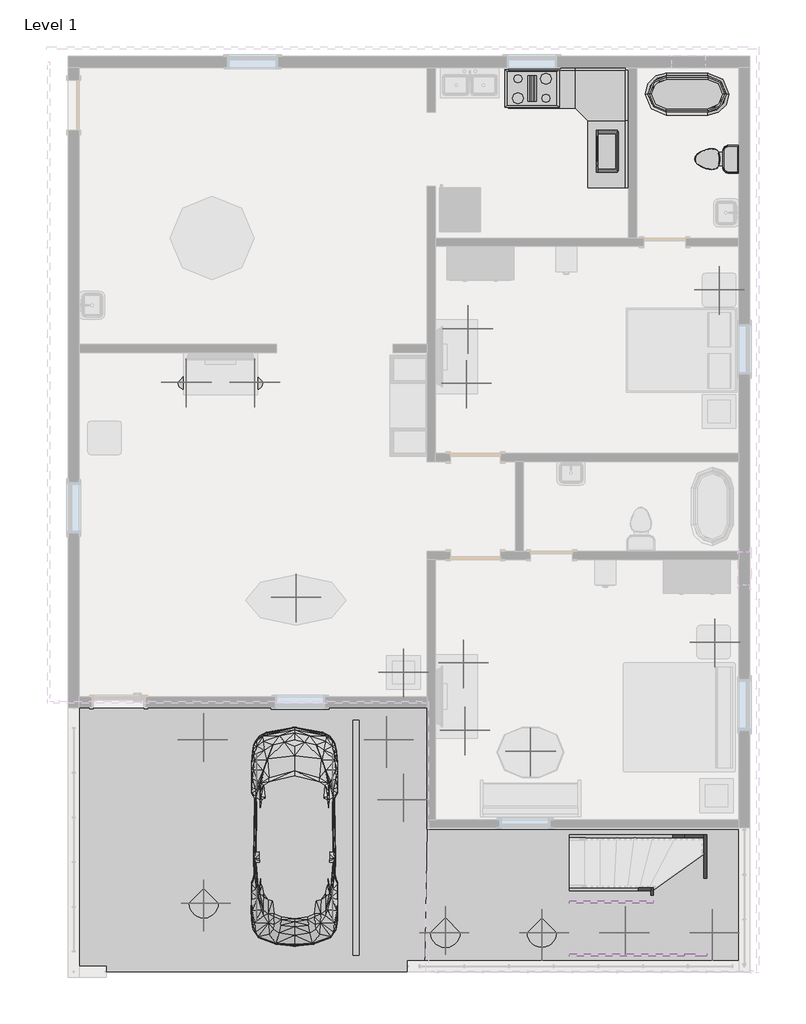
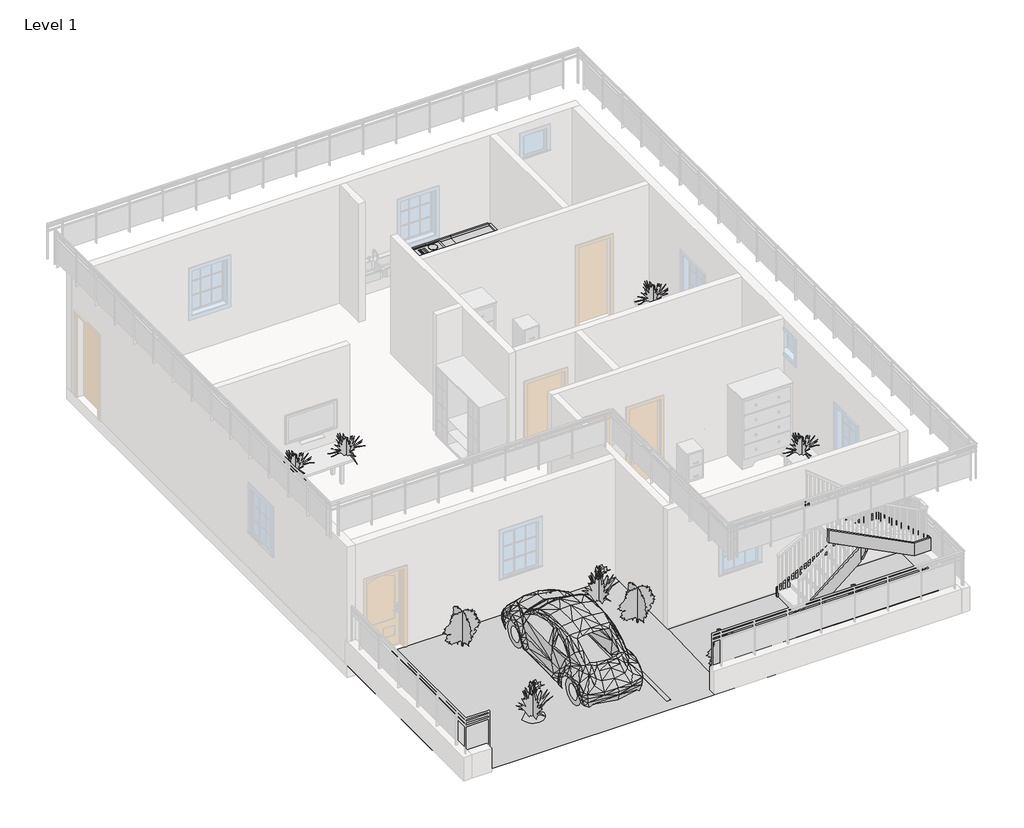
# One storey, part 5 of 5: 19 geographic elements, 8 members, 6 proxies, 3 flow terminals, 1 furniture element.
"""IFC4 building model written with IfcOpenShell, lengths in millimetres."""

from ifc_helpers import new_model, si_unit, frame, origin, place, context, project, spatial, polyline, outline, extrude, triangles, transform, mapped, element, save
from components import proxy_bb1e6e30, proxy_8a8d5ab2, parking_space_9_x_18_90_deg_fdd9e8f5, rpc_beetle_rpc_beetle_3ce7ba48, flow_terminal_accce45a, toilet_domestic_3d_toilet_domestic_3d_f7549cf7, toilet_domestic_3d_toilet_domestic_3d_183bbd19, flow_terminal_b374fae2, furniture_4f0cce40, rpc_plant_tropical_55f6ff97, rpc_plant_tropical_agave_1_5_93a2a214, rpc_plant_tropical_jungle_flame_3_9c4808c2

model = new_model("IFC4")

# Units and contexts
model_context = context("Model", 3, world=origin())
ifc_project = project(units=[si_unit("LENGTHUNIT", "METRE", prefix="MILLI")], contexts=[model_context])

# Site, building, storey
site = spatial("IfcSite", under=ifc_project)
building = spatial("IfcBuilding", under=site)
storey = spatial("IfcBuildingStorey", under=building, Name="Level 1", Elevation=0.0)

# Proxies
placement = place(None, origin())
element("IfcBuildingElementProxy", 1, Name="Building Element Proxy", at=placement, inside=storey, context=model_context, shape_type="Tessellation", body=[
    triangles([(-5791.023848, -19.9366942, 0.0), (-5841.8242355, -2636.1367676, 0.0), (76.3758886, -19.9366942, 0.0), (76.3758886, -2636.1367676, 0.0)], [[1, 2, 4], [4, 3, 1]], closed=False),
])
element("IfcBuildingElementProxy", 2, Name="Building Element Proxy", at=placement, inside=storey, context=model_context, shape_type="Tessellation", body=[
    triangles([(-12318.8236542, 2164.4633778, 0.0), (-12318.8236542, -2636.1367676, 0.0), (-5841.8242355, -2636.1367676, 0.0), (-5791.023848, 2164.4633778, 0.0), (-5791.023848, -19.9366942, 0.0)], [[1, 2, 5], [5, 4, 1], [5, 2, 3]], closed=False),
])
proxy_shape = proxy_bb1e6e30(model_context)
element("IfcBuildingElementProxy", 3, Name="Cook Top-4 Unit : 36\" x 20\"", ObjectType="Cook Top-4 Unit : 36\" x 20\"", at=placement, inside=storey, context=model_context, shape_type="MappedRepresentation", body=[
    mapped(proxy_shape, transform((-3886.0241134, 13416.6633056, 0.0), x_axis=(1.0, 0.0, 0.0), y_axis=(0.0, 1.0, 0.0), z_axis=(0.0, 0.0, 1.0))),
])
proxy_2_shape = proxy_8a8d5ab2(model_context)
element("IfcBuildingElementProxy", 4, Name="Microwave : 30\" x 16\" x 18\"", ObjectType="Microwave : 30\" x 16\" x 18\"", at=placement, inside=storey, context=model_context, shape_type="MappedRepresentation", body=[
    mapped(proxy_2_shape, transform((-2161.3436076, 12773.956183, 0.0), x_axis=(0.0, -1.0000000000000004, 0.0), y_axis=(1.0000000000000004, 0.0, 0.0), z_axis=(0.0, 0.0, 1.0))),
])
parking_space_9_x_18_90_deg_shape = parking_space_9_x_18_90_deg_fdd9e8f5(model_context)
element("IfcBuildingElementProxy", 5, Name="Parking Space : 9' x 18' - 90 deg", ObjectType="Parking Space : 9' x 18' - 90 deg", at=placement, inside=storey, context=model_context, shape_type="MappedRepresentation", body=[
    mapped(parking_space_9_x_18_90_deg_shape, transform((-7086.4241134, -2331.3366944, 0.0), x_axis=(-0.9999999999999999, 0.0, 0.0), y_axis=(0.0, -0.9999999999999999, 0.0), z_axis=(0.0, 0.0, 1.0))),
])
rpc_beetle_rpc_beetle_shape = rpc_beetle_rpc_beetle_3ce7ba48(model_context)
element("IfcBuildingElementProxy", 6, Name="RPC Beetle : RPC Beetle", ObjectType="RPC Beetle : RPC Beetle", at=placement, inside=storey, context=model_context, shape_type="MappedRepresentation", body=[
    mapped(rpc_beetle_rpc_beetle_shape, transform((-8204.0241134, -1416.9366944, 0.0), x_axis=(1.0, 0.0, 0.0), y_axis=(0.0, 1.0, 0.0), z_axis=(0.0, 0.0, 1.0))),
])

# Flow terminals
flow_terminal_shape = flow_terminal_accce45a(model_context)
element("IfcFlowTerminal", 7, ObjectType="Floor Drain - Round : 5\" Strainer - 2\" Drain", at=placement, inside=storey, context=model_context, shape_type="MappedRepresentation", body=[
    mapped(flow_terminal_shape, transform((-412.5741134, 12654.6633056, 0.0), x_axis=(1.0, 0.0, 0.0), y_axis=(0.0, 1.0, 0.0), z_axis=(0.0, 0.0, 1.0))),
])
toilet_domestic_3d_toilet_domestic_3d_shape = toilet_domestic_3d_toilet_domestic_3d_f7549cf7(model_context)
toilet_domestic_3d_toilet_domestic_3d_2_shape = toilet_domestic_3d_toilet_domestic_3d_183bbd19(model_context)
element("IfcFlowTerminal", 8, ObjectType="Toilet-Domestic-3D : Toilet-Domestic-3D", at=placement, inside=storey, context=model_context, shape_type="MappedRepresentation", body=[
    mapped(toilet_domestic_3d_toilet_domestic_3d_shape, transform((-621.5201408, 12133.9633056, 0.0), x_axis=(0.0, -1.0000000000000004, 0.0), y_axis=(1.0000000000000004, 0.0, 0.0), z_axis=(0.0, 0.0, 1.0))),
    mapped(toilet_domestic_3d_toilet_domestic_3d_2_shape, transform((-621.5201408, 12133.9633056, 0.0), x_axis=(0.0, -1.0000000000000004, 0.0), y_axis=(1.0000000000000004, 0.0, 0.0), z_axis=(0.0, 0.0, 1.0))),
])
flow_terminal_2_shape = flow_terminal_b374fae2(model_context)
element("IfcFlowTerminal", 9, ObjectType="Tub-Free Standing-3D : 30\" x 60\"", at=placement, inside=storey, context=model_context, shape_type="MappedRepresentation", body=[
    mapped(flow_terminal_2_shape, transform((-1066.6241134, 13315.0633056, 0.0), x_axis=(0.0, 1.0000000000000002, 0.0), y_axis=(-1.0000000000000002, 0.0, 0.0), z_axis=(0.0, 0.0, 1.0))),
])

# Furniture
furniture_shape = furniture_4f0cce40(model_context)
element("IfcFurniture", 10, ObjectType="Work Station Cubicle : 96\" x 96\"", at=placement, inside=storey, context=model_context, shape_type="MappedRepresentation", body=[
    mapped(furniture_shape, transform((-1638.4011058, 13665.9315534, 0.0), x_axis=(0.0, -1.0000000000000004, 0.0), y_axis=(1.0000000000000004, 0.0, 0.0), z_axis=(0.0, 0.0, 1.0))),
])

# Geographic elements
rpc_plant_tropical_shape = rpc_plant_tropical_55f6ff97(model_context)
element("IfcGeographicElement", 11, ObjectType="RPC Plant - Tropical", at=placement, inside=storey, context=model_context, shape_type="MappedRepresentation", body=[
    mapped(rpc_plant_tropical_shape, transform((-6527.6241134, 1580.2633056, 0.0), x_axis=(1.0, 0.0, 0.0), y_axis=(0.0, 1.0, 0.0), z_axis=(0.0, 0.0, 1.0))),
])
element("IfcGeographicElement", 12, ObjectType="RPC Plant - Tropical", at=placement, inside=storey, context=model_context, shape_type="MappedRepresentation", body=[
    mapped(rpc_plant_tropical_shape, transform((-609.4241134, -1924.9366944, 0.0), x_axis=(1.0, 0.0, 0.0), y_axis=(0.0, 1.0, 0.0), z_axis=(0.0, 0.0, 1.0))),
])
element("IfcGeographicElement", 13, ObjectType="RPC Plant - Tropical", at=placement, inside=storey, context=model_context, shape_type="MappedRepresentation", body=[
    mapped(rpc_plant_tropical_shape, transform((-3708.2241134, -1924.9366944, 0.0), x_axis=(1.0, 0.0, 0.0), y_axis=(0.0, 1.0, 0.0), z_axis=(0.0, 0.0, 1.0))),
])
element("IfcGeographicElement", 14, ObjectType="RPC Plant - Tropical", at=placement, inside=storey, context=model_context, shape_type="MappedRepresentation", body=[
    mapped(rpc_plant_tropical_shape, transform((-9855.0241134, -1391.5366944, 0.0), x_axis=(1.0, 0.0, 0.0), y_axis=(0.0, 1.0, 0.0), z_axis=(0.0, 0.0, 1.0))),
])
rpc_plant_tropical_agave_1_5_shape = rpc_plant_tropical_agave_1_5_93a2a214(model_context)
element("IfcGeographicElement", 15, ObjectType="RPC Plant - Tropical : Agave - 1.5'", at=placement, inside=storey, context=model_context, shape_type="MappedRepresentation", body=[
    mapped(rpc_plant_tropical_agave_1_5_shape, transform((-482.4241134, 9759.0633056, 609.6), x_axis=(1.0, 0.0, 0.0), y_axis=(0.0, 1.0, 0.0), z_axis=(0.0, 0.0, 1.0))),
])
element("IfcGeographicElement", 16, ObjectType="RPC Plant - Tropical : Agave - 1.5'", at=placement, inside=storey, context=model_context, shape_type="MappedRepresentation", body=[
    mapped(rpc_plant_tropical_agave_1_5_shape, transform((-5054.4241134, 9047.8633056, 609.6), x_axis=(1.0, 0.0, 0.0), y_axis=(0.0, 1.0, 0.0), z_axis=(0.0, 0.0, 1.0))),
])
element("IfcGeographicElement", 17, ObjectType="RPC Plant - Tropical : Agave - 1.5'", at=placement, inside=storey, context=model_context, shape_type="MappedRepresentation", body=[
    mapped(rpc_plant_tropical_agave_1_5_shape, transform((-5079.8241134, 8057.2633056, 609.6), x_axis=(1.0, 0.0, 0.0), y_axis=(0.0, 1.0, 0.0), z_axis=(0.0, 0.0, 1.0))),
])
element("IfcGeographicElement", 18, ObjectType="RPC Plant - Tropical : Agave - 1.5'", at=placement, inside=storey, context=model_context, shape_type="MappedRepresentation", body=[
    mapped(rpc_plant_tropical_agave_1_5_shape, transform((-558.6241134, 3358.2633056, 609.6), x_axis=(1.0, 0.0, 0.0), y_axis=(0.0, 1.0, 0.0), z_axis=(0.0, 0.0, 1.0))),
])
element("IfcGeographicElement", 19, ObjectType="RPC Plant - Tropical : Agave - 1.5'", at=placement, inside=storey, context=model_context, shape_type="MappedRepresentation", body=[
    mapped(rpc_plant_tropical_agave_1_5_shape, transform((-5130.6241134, 2977.2633056, 660.4), x_axis=(1.0, 0.0, 0.0), y_axis=(0.0, 1.0, 0.0), z_axis=(0.0, 0.0, 1.0))),
])
element("IfcGeographicElement", 20, ObjectType="RPC Plant - Tropical : Agave - 1.5'", at=placement, inside=storey, context=model_context, shape_type="MappedRepresentation", body=[
    mapped(rpc_plant_tropical_agave_1_5_shape, transform((-5105.2241134, 1758.0633056, 660.4), x_axis=(1.0, 0.0, 0.0), y_axis=(0.0, 1.0, 0.0), z_axis=(0.0, 0.0, 1.0))),
])
element("IfcGeographicElement", 21, ObjectType="RPC Plant - Tropical : Agave - 1.5'", at=placement, inside=storey, context=model_context, shape_type="MappedRepresentation", body=[
    mapped(rpc_plant_tropical_agave_1_5_shape, transform((-3911.4241134, 1377.0633056, 736.6), x_axis=(1.0, 0.0, 0.0), y_axis=(0.0, 1.0, 0.0), z_axis=(0.0, 0.0, 1.0))),
])
element("IfcGeographicElement", 22, ObjectType="RPC Plant - Tropical : Agave - 1.5'", at=placement, inside=storey, context=model_context, shape_type="MappedRepresentation", body=[
    mapped(rpc_plant_tropical_agave_1_5_shape, transform((-6222.8241134, 2805.8133056, 609.6), x_axis=(1.0, 0.0, 0.0), y_axis=(0.0, 1.0, 0.0), z_axis=(0.0, 0.0, 1.0))),
])
element("IfcGeographicElement", 23, ObjectType="RPC Plant - Tropical : Agave - 1.5'", at=placement, inside=storey, context=model_context, shape_type="MappedRepresentation", body=[
    mapped(rpc_plant_tropical_agave_1_5_shape, transform((-8178.6241134, 4171.0633056, 685.8), x_axis=(1.0, 0.0, 0.0), y_axis=(0.0, 1.0, 0.0), z_axis=(0.0, 0.0, 1.0))),
])
element("IfcGeographicElement", 24, ObjectType="RPC Plant - Tropical : Agave - 1.5'", at=placement, inside=storey, context=model_context, shape_type="MappedRepresentation", body=[
    mapped(rpc_plant_tropical_agave_1_5_shape, transform((-8927.9241134, 8082.6633056, 660.4), x_axis=(1.0, 0.0, 0.0), y_axis=(0.0, 1.0, 0.0), z_axis=(0.0, 0.0, 1.0))),
])
element("IfcGeographicElement", 25, ObjectType="RPC Plant - Tropical : Agave - 1.5'", at=placement, inside=storey, context=model_context, shape_type="MappedRepresentation", body=[
    mapped(rpc_plant_tropical_agave_1_5_shape, transform((-10172.5241134, 8082.6633056, 660.4), x_axis=(1.0, 0.0, 0.0), y_axis=(0.0, 1.0, 0.0), z_axis=(0.0, 0.0, 1.0))),
])
rpc_plant_tropical_jungle_flame_3_shape = rpc_plant_tropical_jungle_flame_3_9c4808c2(model_context)
element("IfcGeographicElement", 26, ObjectType="RPC Plant - Tropical : Jungle Flame - 3'", at=placement, inside=storey, context=model_context, shape_type="MappedRepresentation", body=[
    mapped(rpc_plant_tropical_jungle_flame_3_shape, transform((-6222.8241134, 488.0633056, 0.0), x_axis=(1.0, 0.0, 0.0), y_axis=(0.0, 1.0, 0.0), z_axis=(0.0, 0.0, 1.0))),
])
element("IfcGeographicElement", 27, ObjectType="RPC Plant - Tropical : Jungle Flame - 3'", at=placement, inside=storey, context=model_context, shape_type="MappedRepresentation", body=[
    mapped(rpc_plant_tropical_jungle_flame_3_shape, transform((-2184.2241134, -1924.9366944, 0.0), x_axis=(1.0, 0.0, 0.0), y_axis=(0.0, 1.0, 0.0), z_axis=(0.0, 0.0, 1.0))),
])
element("IfcGeographicElement", 28, ObjectType="RPC Plant - Tropical : Jungle Flame - 3'", at=placement, inside=storey, context=model_context, shape_type="MappedRepresentation", body=[
    mapped(rpc_plant_tropical_jungle_flame_3_shape, transform((-5460.8241134, -1924.9366944, 0.0), x_axis=(1.0, 0.0, 0.0), y_axis=(0.0, 1.0, 0.0), z_axis=(0.0, 0.0, 1.0))),
])
element("IfcGeographicElement", 29, ObjectType="RPC Plant - Tropical : Jungle Flame - 3'", at=placement, inside=storey, context=model_context, shape_type="MappedRepresentation", body=[
    mapped(rpc_plant_tropical_jungle_flame_3_shape, transform((-9855.0241134, 1580.2633056, 0.0), x_axis=(1.0, 0.0, 0.0), y_axis=(0.0, 1.0, 0.0), z_axis=(0.0, 0.0, 1.0))),
])

# Members
element("IfcMember", 30, ObjectType="Stringer - 2\" Width", at=placement, inside=storey, context=model_context, shape_type="SweptSolid", body=[
    extrude(outline(polyline([(229.639954, -3203.9558053), (0.0, -3203.9558053), (0.0, -2984.1934877), (962.500629, -1116.5386136), (1305.3956453, -1116.5386136), (229.639954, -3203.9558053)])), frame((0.0, -197.7366944, 0.0), z_axis=(0.0, 1.0, 0.0), x_axis=(0.0, 0.0, 1.0)), (0.0, 0.0, 1.0), 50.8),
])
element("IfcMember", 31, ObjectType="Stringer - 2\" Width", at=placement, inside=storey, context=model_context, shape_type="SweptSolid", body=[
    extrude(outline(polyline([(-1116.5386136, -197.7366944), (-1116.5386136, -146.9366944), (-761.8241134, -146.9366944), (-761.8241134, -197.7366944), (-1116.5386136, -197.7366944)])), frame((0.0, 0.0, 962.500629), z_axis=(0.0, 0.0, 1.0), x_axis=(1.0, 0.0, 0.0)), (0.0, 0.0, 1.0), 342.8950162),
])
element("IfcMember", 32, ObjectType="Stringer - 2\" Width", at=placement, inside=storey, context=model_context, shape_type="SweptSolid", body=[
    extrude(outline(polyline([(-146.9366944, 1289.0952212), (-146.9366944, 1000.5956453), (-316.4591773, 1000.5956453), (-2305.9366944, 1638.9682298), (-2305.9366944, 1969.9972697), (-2268.9565771, 1969.9972697), (-146.9366944, 1289.0952212)])), frame((-761.8241134, 0.0, 0.0), z_axis=(1.0, 0.0, 0.0), x_axis=(0.0, 1.0, 0.0)), (0.0, 0.0, 1.0), 50.8),
])
element("IfcMember", 33, ObjectType="Stringer - 2\" Width", at=placement, inside=storey, context=model_context, shape_type="SweptSolid", body=[
    extrude(outline(polyline([(-711.0241134, -2305.9366944), (-711.0241134, -2356.7366944), (-1116.5386136, -2356.7366944), (-1116.5386136, -2305.9366944), (-711.0241134, -2305.9366944)])), frame((0.0, 0.0, 1649.8904473), z_axis=(0.0, 0.0, 1.0), x_axis=(1.0, 0.0, 0.0)), (0.0, 0.0, 1.0), 320.1068224),
])
element("IfcMember", 34, ObjectType="Stringer - 2\" Width", at=placement, inside=storey, context=model_context, shape_type="SweptSolid", body=[
    extrude(outline(polyline([(1649.8904473, -1116.5386136), (1969.9972697, -1116.5386136), (3045.7529609, -3203.9558053), (2725.6461385, -3203.9558053), (1649.8904473, -1116.5386136)])), frame((0.0, -2356.7366944, 0.0), z_axis=(0.0, 1.0, 0.0), x_axis=(0.0, 0.0, 1.0)), (0.0, 0.0, 1.0), 50.8),
])
element("IfcMember", 35, ObjectType="Stringer - 2\" Width", at=placement, inside=storey, context=model_context, shape_type="SweptSolid", body=[
    extrude(outline(polyline([(176.1764461, -3203.9558053), (0.0, -3203.9558053), (0.0, -2937.6941607), (987.1410923, -1727.0241134), (1380.418648, -1727.0241134), (176.1764461, -3203.9558053)])), frame((0.0, -1162.9366944, 0.0), z_axis=(0.0, 1.0, 0.0), x_axis=(0.0, 0.0, 1.0)), (0.0, 0.0, 1.0), 50.8),
])
element("IfcMember", 36, ObjectType="Stringer - 2\" Width", at=placement, inside=storey, context=model_context, shape_type="SweptSolid", body=[
    extrude(outline(polyline([(-1112.1366944, 1573.2682978), (-1112.1366944, 1028.5617647), (-1146.3789117, 1028.5617647), (-1340.7366944, 1360.465107), (-1340.7366944, 1926.1409689), (-1318.7738118, 1926.1409689), (-1112.1366944, 1573.2682978)])), frame((-1727.0241134, 0.0, 0.0), z_axis=(1.0, 0.0, 0.0), x_axis=(0.0, 1.0, 0.0)), (0.0, 0.0, 1.0), 50.8),
])
element("IfcMember", 37, ObjectType="Stringer - 2\" Width", at=placement, inside=storey, context=model_context, shape_type="SweptSolid", body=[
    extrude(outline(polyline([(1532.8634131, -1676.2241134), (1926.1409689, -1676.2241134), (3171.8038432, -3203.9558053), (2778.5262875, -3203.9558053), (1532.8634131, -1676.2241134)])), frame((0.0, -1391.5366944, 0.0), z_axis=(0.0, 1.0, 0.0), x_axis=(0.0, 0.0, 1.0)), (0.0, 0.0, 1.0), 50.8),
])

save(model, "model.ifc")

# Revit data of these elements
# Type "Cook Top-4 Unit : 36\" x 20\""
#   Assembly Code = "E1090400"
#   Depth = 2' - 0"
#   Width = 3' - 0"
#   Burner Material = Steel, Chrome Plated
#   Cooktop Material = Steel, Polished
#   Default Elevation = 0
# Type "Microwave : 30\" x 16\" x 18\""
#   Assembly Code = "E1090400"
#   Depth = 1' - 4"
#   Height = 1' - 6"
#   Width = 2' - 6"
#   Microwave Material = Laminate, Linen, Matte
#   Default Elevation = 0
# Type "Parking Space : 9' x 18' - 90 deg"
#   Angle = 90.00°
#   Parking Length = 18' - 0"
#   Parking Width = 9' - 0"
#   pl = 14' - 0"
#   pw = 7' - 0"
# Type "RPC Beetle : RPC Beetle"
#   built-in parameter 1005195 = "RPC-16-0U6E-L4EG-ENH1-J3KF-SVEL-0TX4-C0"
#   Height = 0
# Type "Floor Drain - Round : 5\" Strainer - 2\" Drain"
#   WFU = 2
#   Strainer Height = 0' - 3 1/4"
#   Strainer Radius = 0' - 2 1/2"
#   Strainer Diameter = 0' - 5"
#   Radius 6 = 0' - 0 5/8"
#   Radius 5 = 0' - 1 1/4"
#   Radius 4 = 0' - 1 7/8"
#   Radius 2 = 0' - 3.04167"
#   Radius 1 = 0' - 2.02083"
#   Radius 3 = 0' - 2 1/32"
#   Pipe Radius = 1"
#   Pipe Diameter = 2"
#   Height 2 = 0' - 0.725"
#   Height 1 = 0' - 1 13/16"
#   Body Radius = 0' - 4 1/16"
#   Body Height = 0' - 3 5/8"
#   Body Diameter = 0' - 8 1/8"
#   Drain Material = none
#   HWFU = 0
#   Default Elevation = 0
#   CWFU = 0
# Type "Toilet-Domestic-3D : Toilet-Domestic-3D"
#   Assembly Code = "D2010110"
#   Toilet - Bowl/Basin Material = Porcelain, Linen
#   Toilet - Seat Material = Laminate, Linen, Matte
#   Default Elevation = 0
# Type "Tub-Free Standing-3D : 30\" x 60\""
#   Assembly Code = "D2010110"
#   Height = 1' - 6"
#   Length = 5' - 0"
#   Width = 2' - 6"
#   Tub Material = Porcelain, Ivory
#   Default Elevation = 0
# Type "Work Station Cubicle : 96\" x 96\""
#   Assembly Code = "E2020"
#   Desktop Height = 2' - 6"
#   Desktop1 Width = 2' - 3"
#   Desktop2 Width = 2' - 3"
#   Panel Height = 2' - 8"
#   Panel1 Length = 4' - 0"
#   Panel2 Length = 4' - 0"
#   Cube Panel Material = Textile - Light Gray
#   Work Top Material = Laminate, Ivory, Matte
#   Default Elevation = 0
# Type "RPC Plant - Tropical"
#   built-in parameter 1005198 = "{2, 15},{39, RPC-16-FWM5-GM7X-C67P-4000-ST1L-LVER-AU},{1, 0},{1, 0},{2, 13},{1, 8},{5, Color},{1, 0},{1, 0},{3, 0.8},{3, 0.8},{3, 0.8},{1, 8},{7, BBoxMin},{1, 0},{1, 0},{1, 0},{1, 0},{1, 0},{1, 8},{7, BBoxMax},{1, 0},{1, 0},{1, 0},{1, 0},{1, 0},{2, 11},{9, RPCTypeId},{1, 0},{1, 0},{39, RPC-16-FWM5-GM7X-C67P-4000-ST1L-LVER-AU},{1, 6},{14, RPCPlantHeight},{1, 0},{1, 0},{1, 3},{2, 11},{7, keyword},{1, 0},{1, 0},{35, :RPCs:Shrubs [General]:Geometry:RPC},{2, 11},{8, category},{1, 0},{1, 0},{16, Shrubs [General]},{2, 11},{12, LocalizedUID},{1, 0},{1, 0},{10, Crane Lily},{2, 14},{6, Height},{1, 0},{1, 0},{1, 3},{1, 2},{16, Cast Reflections},{1, 0},{1, 0},{1, 0},{1, 2},{12, Cast Shadows},{1, 0},{1, 0},{1, 1},{1, 2},{9, Lock View},{1, 0},{1, 0},{1, 0},{1, 4},{5, ViewC},{1, 0},{1, 0},{1, 0},{21, assetlibrary_base.fbx},{1, 5},"
#   built-in parameter 1005195 = "RPC-16-FWM5-GM7X-C67P-4000-ST1L-LVER-AU"
#   Assembly Code = "G2050500"
#   Height = 3' - 0"
#   Default Elevation = 0
# Type "RPC Plant - Tropical : Agave - 1.5'"
#   built-in parameter 1005198 = "{2, 15},{39, RPC-16-G1GJ-63FX-7K5P-N000-ST1L-LVER-AU},{1, 0},{1, 0},{2, 13},{1, 8},{5, Color},{1, 0},{1, 0},{3, 0.8},{3, 0.8},{3, 0.8},{1, 8},{7, BBoxMin},{1, 0},{1, 0},{1, 0},{1, 0},{1, 0},{1, 8},{7, BBoxMax},{1, 0},{1, 0},{1, 0},{1, 0},{1, 0},{2, 11},{9, RPCTypeId},{1, 0},{1, 0},{39, RPC-16-G1GJ-63FX-7K5P-N000-ST1L-LVER-AU},{1, 6},{14, RPCPlantHeight},{1, 0},{1, 0},{3, 1.5},{2, 11},{7, keyword},{1, 0},{1, 0},{35, :RPCs:Plants [General]:Geometry:RPC},{2, 11},{8, category},{1, 0},{1, 0},{16, Plants [General]},{2, 11},{12, LocalizedUID},{1, 0},{1, 0},{5, Agave},{2, 14},{6, Height},{1, 0},{1, 0},{3, 1.5},{1, 2},{16, Cast Reflections},{1, 0},{1, 0},{1, 0},{1, 2},{12, Cast Shadows},{1, 0},{1, 0},{1, 1},{1, 2},{9, Lock View},{1, 0},{1, 0},{1, 0},{1, 4},{5, ViewC},{1, 0},{1, 0},{1, 0},{21, assetlibrary_base.fbx},{1, 5},"
#   built-in parameter 1005195 = "RPC-16-G1GJ-63FX-7K5P-N000-ST1L-LVER-AU"
#   Type Comments = "Agave"
#   Assembly Code = "G2050500"
#   Height = 1' - 6"
#   Default Elevation = 0
# Type "RPC Plant - Tropical : Jungle Flame - 3'"
#   built-in parameter 1005198 = "{2, 15},{39, RPC-16-FUVJ-JWG0-MWGK-8000-ST1L-LVER-AU},{1, 0},{1, 0},{2, 13},{1, 8},{5, Color},{1, 0},{1, 0},{3, 0.8},{3, 0.8},{3, 0.8},{1, 8},{7, BBoxMin},{1, 0},{1, 0},{1, 0},{1, 0},{1, 0},{1, 8},{7, BBoxMax},{1, 0},{1, 0},{1, 0},{1, 0},{1, 0},{2, 11},{9, RPCTypeId},{1, 0},{1, 0},{39, RPC-16-FUVJ-JWG0-MWGK-8000-ST1L-LVER-AU},{1, 6},{14, RPCPlantHeight},{1, 0},{1, 0},{1, 3},{2, 11},{7, keyword},{1, 0},{1, 0},{35, :RPCs:Shrubs [General]:Geometry:RPC},{2, 11},{8, category},{1, 0},{1, 0},{16, Shrubs [General]},{2, 11},{12, LocalizedUID},{1, 0},{1, 0},{12, Jungle Flame},{2, 14},{6, Height},{1, 0},{1, 0},{1, 3},{1, 2},{16, Cast Reflections},{1, 0},{1, 0},{1, 0},{1, 2},{12, Cast Shadows},{1, 0},{1, 0},{1, 1},{1, 2},{9, Lock View},{1, 0},{1, 0},{1, 0},{1, 4},{5, ViewC},{1, 0},{1, 0},{1, 0},{21, assetlibrary_base.fbx},{1, 5},"
#   built-in parameter 1005195 = "RPC-16-FUVJ-JWG0-MWGK-8000-ST1L-LVER-AU"
#   Type Comments = "Jungle Flame"
#   Assembly Code = "G2050500"
#   Height = 3' - 0"
#   Default Elevation = 0
# Elements 1, 2 (IfcBuildingElementProxy)
#   Material = Plant
#   Phase Created = New Construction
# Element 3 (IfcBuildingElementProxy, "Cook Top-4 Unit : 36\" x 20\"")
#   Phase Created = New Construction
#   Materials on its faces: "Steel, Chrome Plated", "Steel, Polished"
# Element 4 (IfcBuildingElementProxy, "Microwave : 30\" x 16\" x 18\"")
#   Phase Created = New Construction
#   Materials on its faces: "Laminate, Linen, Matte", "Glass"
# Element 5 (IfcBuildingElementProxy, "Parking Space : 9' x 18' - 90 deg")
#   Phase Created = New Construction
#   Materials on its faces: "Parking Stripe"
# Element 6 (IfcBuildingElementProxy, "RPC Beetle : RPC Beetle")
#   Phase Created = New Construction
# Element 7 (IfcFlowTerminal, "Floor Drain - Round : 5\" Strainer - 2\" Drain")
#   Mark = "6"
#   Phase Created = New Construction
# Element 8 (IfcFlowTerminal, "Toilet-Domestic-3D : Toilet-Domestic-3D")
#   Mark = "4"
#   Phase Created = New Construction
#   Materials on its faces: "Porcelain, Linen", "Laminate, Linen, Matte"
# Element 9 (IfcFlowTerminal, "Tub-Free Standing-3D : 30\" x 60\"")
#   Mark = "3"
#   Phase Created = New Construction
#   Materials on its faces: "Porcelain, Ivory"
# Element 10 (IfcFurniture, "Work Station Cubicle : 96\" x 96\"")
#   Phase Created = New Construction
#   Materials on its faces: "Textile - Light Gray", "Laminate, Ivory, Matte"
# Elements 11, 12, 13, 14 (IfcGeographicElement, "RPC Plant - Tropical")
#   Phase Created = New Construction
# Elements 15, 16, 17, 18, 19, 20, 21, 22, 23, 24, 25 (IfcGeographicElement, "RPC Plant - Tropical : Agave - 1.5'")
#   Phase Created = New Construction
# Elements 26, 27, 28, 29 (IfcGeographicElement, "RPC Plant - Tropical : Jungle Flame - 3'")
#   Phase Created = New Construction
# Elements 30, 31, 32, 33, 34, 35, 36, 37 (IfcMember, "Stringer - 2\" Width")
#   Phase Created = New Construction
# Materials
#   "Steel, Chrome Plated": class "Metal", colour RGB 17 17 17, transparency 0, Description = "Chromiuim plated steel", Cost = 0
#   "Steel, Polished": class "Metal", colour RGB 57 57 57, transparency 0, Description = "Polished steel", Cost = 0
#   "Laminate, Linen, Matte": class "Plastic", colour RGB 249 239 230, transparency 0, Description = "Plastic Laminate - Linen, Matte", Cost = 0
#   "Porcelain, Linen": class "Ceramic", colour RGB 249 239 230, transparency 0, Description = "Porcelain, linen", Cost = 0
#   "Porcelain, Ivory": class "Ceramic", colour RGB 247 247 239, transparency 0, Description = "Porcelain, ivory", Cost = 0
#   "Textile - Light Gray": class "Fabric", colour RGB 204 204 204, transparency 0
#   "Laminate, Ivory, Matte": class "Plastic", colour RGB 247 247 239, transparency 0, Description = "Plastic Laminate - Ivory, Matte", Cost = 0
#   "Plant": class "Generic", colour RGB 0 0 0, transparency 0, Description = "physical material", Cost = 0
#   "Glass": class "Glass", colour RGB 0 128 192, transparency 0.75, Description = "Soda Lime Glass", Cost = 0
#   "Parking Stripe": class "Paint", colour RGB 250 250 91, transparency 0
